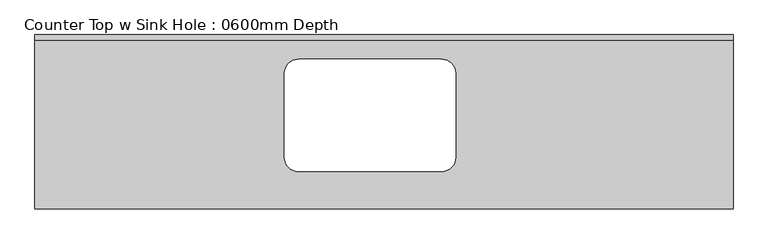
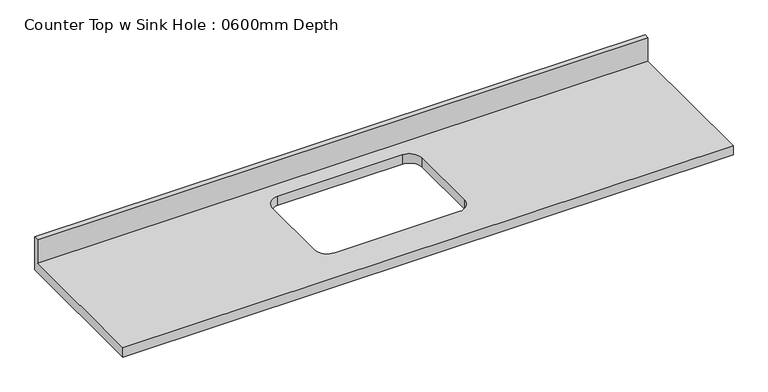
"""IFC4 building model written with IfcOpenShell, lengths in millimetres: furniture geometry, Counter Top w Sink Hole : 0600mm Depth."""

from ifc_helpers import new_model, si_unit, frame, origin, place, context, project, spatial, polyline, circle_curve, source, transform, mapped, element, save
from ifc_brep_helpers import plane_surface, revolved_surface, advanced_brep


def counter_top_w_sink_hole_0600mm_depth_f226a61d(model_context):
    return source(origin(), model_context, "Body", "AdvancedBrep", [
        advanced_brep(
        [(-1200.4622951, -624.68125, 900.1125), (1299.8502049, -624.68125, 900.1125), (1299.8502049, -19.05, 900.1125), (-1200.4622951, -19.05, 900.1125), (-255.8997951, -87.3125, 900.1125), (255.2752049, -87.3125, 900.1125), (306.0752049, -138.1125, 900.1125), (306.0752049, -439.7375, 900.1125), (255.2752049, -490.5375, 900.1125), (-255.8997951, -490.5375, 900.1125), (-306.6997951, -439.7375, 900.1125), (-306.6997951, -138.1125, 900.1125), (1299.8502049, 0.0, 860.425), (1299.8502049, -624.68125, 860.425), (-1200.4622951, -624.68125, 860.425), (-1200.4622951, 0.0, 860.425), (255.2752049, -87.3125, 860.425), (-255.8997951, -87.3125, 860.425), (-306.6997951, -138.1125, 860.425), (-306.6997951, -439.7375, 860.425), (-255.8997951, -490.5375, 860.425), (255.2752049, -490.5375, 860.425), (306.0752049, -439.7375, 860.425), (306.0752049, -138.1125, 860.425), (-1200.4622951, 0.0, 1001.7125), (1299.8502049, 0.0, 1001.7125), (-1200.4622951, -19.05, 1001.7125), (1299.8502049, -19.05, 1001.7125)],
        [
            (0, 1),
            (1, 2),
            (2, 3),
            (3, 0),
            (4, 5),
            (5, 6, circle_curve(frame((255.2752049, -138.1125, 900.1125), z_axis=(0.0, 0.0, -1.0), x_axis=(1.0, 0.0, 0.0)), 50.8)),
            (6, 7),
            (7, 8, circle_curve(frame((255.2752049, -439.7375, 900.1125), z_axis=(0.0, 0.0, -1.0), x_axis=(1.0, 0.0, 0.0)), 50.8)),
            (8, 9),
            (9, 10, circle_curve(frame((-255.8997951, -439.7375, 900.1125), z_axis=(0.0, 0.0, -1.0), x_axis=(1.0, 0.0, 0.0)), 50.8)),
            (10, 11),
            (11, 4, circle_curve(frame((-255.8997951, -138.1125, 900.1125), z_axis=(0.0, 0.0, -1.0), x_axis=(1.0, 0.0, 0.0)), 50.8)),
            (12, 13),
            (13, 14),
            (14, 15),
            (15, 12),
            (16, 17),
            (17, 18, circle_curve(frame((-255.8997951, -138.1125, 860.425), z_axis=(0.0, 0.0, 1.0), x_axis=(1.0, 0.0, 0.0)), 50.8)),
            (18, 19),
            (19, 20, circle_curve(frame((-255.8997951, -439.7375, 860.425), z_axis=(0.0, 0.0, 1.0), x_axis=(1.0, 0.0, 0.0)), 50.8)),
            (20, 21),
            (21, 22, circle_curve(frame((255.2752049, -439.7375, 860.425), z_axis=(0.0, 0.0, 1.0), x_axis=(1.0, 0.0, 0.0)), 50.8)),
            (22, 23),
            (23, 16, circle_curve(frame((255.2752049, -138.1125, 860.425), z_axis=(0.0, 0.0, 1.0), x_axis=(1.0, 0.0, 0.0)), 50.8)),
            (15, 24),
            (24, 25),
            (25, 12),
            (14, 0),
            (3, 26),
            (26, 24),
            (13, 1),
            (25, 27),
            (27, 2),
            (26, 27),
            (4, 17),
            (16, 5),
            (11, 18),
            (10, 19),
            (9, 20),
            (8, 21),
            (7, 22),
            (6, 23),
        ],
        [
            plane_surface(frame((-1200.4622951, 0.0, 900.1125), z_axis=(0.0, 0.0, 1.0), x_axis=(-1.0, 0.0, 0.0))),
            plane_surface(frame((-1200.4622951, 0.0, 860.425), z_axis=(0.0, 0.0, -1.0), x_axis=(1.0, 0.0, 0.0))),
            plane_surface(frame((1299.8502049, 0.0, 900.1125), z_axis=(0.0, 1.0, 0.0), x_axis=(0.0, 0.0, -1.0))),
            plane_surface(frame((-1200.4622951, 0.0, 900.1125), z_axis=(-1.0, 0.0, 0.0), x_axis=(0.0, 0.0, -1.0))),
            plane_surface(frame((-1200.4622951, -624.68125, 900.1125), z_axis=(0.0, -1.0, 0.0), x_axis=(0.0, 0.0, -1.0))),
            plane_surface(frame((1299.8502049, -624.68125, 900.1125), z_axis=(1.0, 0.0, 0.0), x_axis=(0.0, 0.0, -1.0))),
            plane_surface(frame((-1200.4622951, 0.0, 1001.7125), z_axis=(0.0, 0.0, 1.0), x_axis=(0.0, -1.0, 0.0))),
            plane_surface(frame((-1200.4622951, -19.05, 1001.7125), z_axis=(0.0, -1.0, 0.0), x_axis=(0.0, 0.0, -1.0))),
            plane_surface(frame((255.2752049, -87.3125, 900.1125), z_axis=(0.0, -1.0, 0.0), x_axis=(0.0, 0.0, -1.0))),
            revolved_surface(polyline([(-205.0997951, -138.1125, 900.1125), (-205.0997951, -138.1125, 860.425)]), (-255.8997951, -138.1125, 860.425), (0.0, 0.0, 1.0)),
            plane_surface(frame((-306.6997951, -138.1125, 900.1125), z_axis=(1.0, 0.0, 0.0), x_axis=(0.0, 0.0, -1.0))),
            revolved_surface(polyline([(-205.0997951, -439.7375, 900.1125), (-205.0997951, -439.7375, 860.425)]), (-255.8997951, -439.7375, 860.425), (0.0, 0.0, 1.0)),
            plane_surface(frame((-255.8997951, -490.5375, 900.1125), z_axis=(0.0, 1.0, 0.0), x_axis=(0.0, 0.0, -1.0))),
            revolved_surface(polyline([(306.0752049, -439.7375, 900.1125), (306.0752049, -439.7375, 860.425)]), (255.2752049, -439.7375, 860.425), (0.0, 0.0, 1.0)),
            plane_surface(frame((306.0752049, -439.7375, 900.1125), z_axis=(-1.0, 0.0, 0.0), x_axis=(0.0, 0.0, -1.0))),
            revolved_surface(polyline([(306.0752049, -138.1125, 900.1125), (306.0752049, -138.1125, 860.425)]), (255.2752049, -138.1125, 860.425), (0.0, 0.0, 1.0)),
        ],
        [
            (0, [[1, 2, 3, 4], [5, 6, 7, 8, 9, 10, 11, 12]]),
            (1, [[13, 14, 15, 16], [17, 18, 19, 20, 21, 22, 23, 24]]),
            (2, [[-16, 25, 26, 27]]),
            (3, [[-15, 28, -4, 29, 30, -25]]),
            (4, [[-1, -28, -14, 31]]),
            (5, [[-13, -27, 32, 33, -2, -31]]),
            (6, [[-30, 34, -32, -26]]),
            (7, [[-34, -29, -3, -33]]),
            (8, [[35, -17, 36, -5]]),
            (9, [[-35, -12, 37, -18]]),
            (10, [[-37, -11, 38, -19]]),
            (11, [[-38, -10, 39, -20]]),
            (12, [[-39, -9, 40, -21]]),
            (13, [[-40, -8, 41, -22]]),
            (14, [[-41, -7, 42, -23]]),
            (15, [[-36, -24, -42, -6]]),
        ],
    ),
    ])


if __name__ == "__main__":
    model = new_model("IFC4")
    model_context = context("Model", 3, world=origin())
    ifc_project = project(units=[si_unit("LENGTHUNIT", "METRE", prefix="MILLI")], contexts=[model_context])
    site = spatial("IfcSite", under=ifc_project)
    building = spatial("IfcBuilding", under=site)
    placement = place(None, origin())
    counter_top_w_sink_hole_0600mm_depth_shape = counter_top_w_sink_hole_0600mm_depth_f226a61d(model_context)
    element("IfcFurniture", 1, ObjectType="Counter Top w Sink Hole : 0600mm Depth", at=placement, inside=building, context=model_context, shape_type="MappedRepresentation", body=[
        mapped(counter_top_w_sink_hole_0600mm_depth_shape, transform((0.0, 0.0, 0.0), x_axis=(1.0, 0.0, 0.0), y_axis=(0.0, 1.0, 0.0), z_axis=(0.0, 0.0, 1.0))),
    ])
    save(model, "model.ifc")

# Revit data of these elements
# Type "Counter Top w Sink Hole : 0600mm Depth"
#   Assembly Code = "C1030400"
#   Counter Thickness = 0' - 1 9/16"
#   Depth = 2' - 0 19/32"
#   Height = 2' - 11 7/16"
#   Length [instance default] = 8' - 2 7/16"
#   Sink Location [instance default] = 3' - 11 1/4"
#   Sink Location To Wall [instance default] = 0' - 3 15/16"
#   Sink Opening Depth [instance default] = 1' - 2 7/8"
#   Sink Opening Width [instance default] = 1' - 11 1/8"
#   Counter Top Material = none
#   Default Elevation = 0
# Element 1 (IfcFurniture, "Counter Top w Sink Hole : 0600mm Depth")
#   Materials on its faces: "Counter Top"
# Materials
#   "Counter Top": class "Wood", colour RGB 226 177 128, transparency 0
